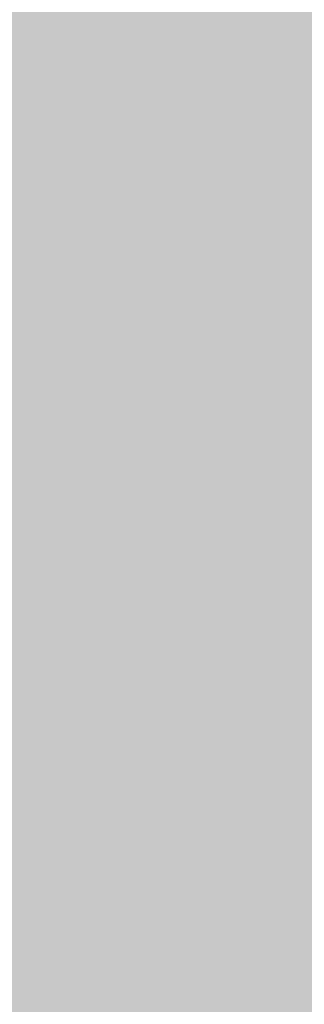
# Model space of a CAD drawing. Units: millimetres. Extents: x -22994 to 29398, y -19990 to 20176.
# Tile 81 of 135: x 225.814 to 226.355, y 85.199 to 87.071. Entities that reach past the tile are written whole.
import ezdxf
from ezdxf import colors
from ezdxf.entities.mleader import LeaderData, LeaderLine
from ezdxf.math import Vec2, Vec3

# ---------------------------------------------------------------- set-up
doc = ezdxf.new("R2010")
doc.units = ezdxf.units.MM
doc.header["$MEASUREMENT"] = 0
doc.layers.add('M-ANNO-TEXT', color=7, linetype='Continuous', lineweight=25)
doc.layers.add('M-DIMS', color=2, linetype='Continuous', lineweight=18)
doc.styles.get("Standard").update_dxf_attribs({"font": 'arial.ttf'})
doc.dimstyles.get("Standard").update_dxf_attribs({"dimtxt": 0.18, "dimasz": 10000, "dimexe": 0.18, "dimexo": 0.0625, "dimgap": 0.09, "dimtad": 0, "dimtih": 1, "dimtoh": 1, "dimdec": 0, "dimzin": 0, "dimdsep": 46, "dimtxsty": 'Standard', "dimcen": 0.09, "dimadec": 0, "dimazin": 0, "dimtfac": 1, "dimtdec": 0, "dimtofl": 0, "dimtmove": 0, "dimatfit": 3, "dimfxl": 1, "dimtolj": 1, "dimtzin": 0, "dimlwd": 30, "dimarcsym": 0})

# ---------------------------------------------------------------- blocks, each defined once
blk = doc.blocks.new('*D2')
at = {"layer": 'Defpoints', "color": 0, "transparency": 16777216}
for p in [(6.6773, 10.2713), (290.852, 10.2713), (290.852, -5.0787)]:
    blk.add_point(p, dxfattribs=at)
at = {"layer": 'M-DIMS', "color": 0, "lineweight": -2, "transparency": 16777216}
for p, q in [((6.6773, 10.2088), (6.6773, -5.2587)), ((290.852, 10.2088), (290.852, -5.2587))]:
    blk.add_line(p, q, dxfattribs=at)
at = {"layer": 'M-DIMS', "color": 0, "lineweight": 30, "transparency": 16777216}
for p, q in [((-9993.3227, -5.0787), (-19993.3227, -5.0787)), ((10290.852, -5.0787), (20290.852, -5.0787))]:
    blk.add_line(p, q, dxfattribs=at)
at = {"layer": 'M-DIMS', "color": 0, "transparency": 16777216}
for points in [[(-9993.3227, 1661.5879), (-9993.3227, -1671.7454), (6.6773, -5.0787)], [(10290.852, 1661.5879), (10290.852, -1671.7454), (290.852, -5.0787)]]:
    blk.add_solid(points, dxfattribs=at)
at = {"layer": 'M-DIMS', "color": 0, "transparency": 16777216, "insert": (148.7647, -5.0787), "char_height": 0.18, "attachment_point": 5}
blk.add_mtext('\\A1;284.2', dxfattribs=at)
blk = doc.blocks.new('*D3')
at = {"layer": 'Defpoints', "color": 0, "transparency": 16777216}
for p in [(110.2647, 204.1654), (110.2647, 176.3662), (95.8327, 127.967)]:
    blk.add_point(p, dxfattribs=at)
at = {"layer": 'M-DIMS', "color": 0, "lineweight": -2, "transparency": 16777216}
for p, q in [((95.8327, 128.0295), (95.8327, 204.3454)), ((110.2647, 176.4287), (110.2647, 204.3454))]:
    blk.add_line(p, q, dxfattribs=at)
at = {"layer": 'M-DIMS', "color": 0, "lineweight": 30, "transparency": 16777216}
for p, q in [((-9904.1673, 204.1654), (-19904.1673, 204.1654)), ((10110.2647, 204.1654), (20110.2647, 204.1654))]:
    blk.add_line(p, q, dxfattribs=at)
at = {"layer": 'M-DIMS', "color": 0, "transparency": 16777216}
for points in [[(-9904.1673, 1870.8321), (-9904.1673, -1462.5013), (95.8327, 204.1654)], [(10110.2647, 1870.8321), (10110.2647, -1462.5013), (110.2647, 204.1654)]]:
    blk.add_solid(points, dxfattribs=at)
at = {"layer": 'M-DIMS', "color": 0, "transparency": 16777216, "insert": (103.0487, 204.1654), "char_height": 0.18, "attachment_point": 5}
blk.add_mtext('\\A1;14.432', dxfattribs=at)
blk = doc.blocks.new('*D4')
at = {"layer": 'Defpoints', "color": 0, "transparency": 16777216}
for p in [(116.2647, 204.1654), (110.2647, 176.3662), (116.2647, 176.3662)]:
    blk.add_point(p, dxfattribs=at)
at = {"layer": 'M-DIMS', "color": 0, "lineweight": -2, "transparency": 16777216}
for p, q in [((110.2647, 176.4287), (110.2647, 204.3454)), ((116.2647, 176.4287), (116.2647, 204.3454))]:
    blk.add_line(p, q, dxfattribs=at)
at = {"layer": 'M-DIMS', "color": 0, "lineweight": 30, "transparency": 16777216}
for p, q in [((-9889.7353, 204.1654), (-19889.7353, 204.1654)), ((10116.2647, 204.1654), (20116.2647, 204.1654))]:
    blk.add_line(p, q, dxfattribs=at)
at = {"layer": 'M-DIMS', "color": 0, "transparency": 16777216}
for points in [[(-9889.7353, 1870.8321), (-9889.7353, -1462.5013), (110.2647, 204.1654)], [(10116.2647, 1870.8321), (10116.2647, -1462.5013), (116.2647, 204.1654)]]:
    blk.add_solid(points, dxfattribs=at)
at = {"layer": 'M-DIMS', "color": 0, "transparency": 16777216, "insert": (113.2647, 204.1654), "char_height": 0.18, "attachment_point": 5}
blk.add_mtext('\\A1;6', dxfattribs=at)
blk = doc.blocks.new('*D5')
at = {"layer": 'Defpoints', "color": 0, "transparency": 16777216}
for p in [(181.2647, 204.1654), (116.2647, 176.3662), (181.2647, 176.3662)]:
    blk.add_point(p, dxfattribs=at)
at = {"layer": 'M-DIMS', "color": 0, "lineweight": -2, "transparency": 16777216}
for p, q in [((116.2647, 176.4287), (116.2647, 204.3454)), ((181.2647, 176.4287), (181.2647, 204.3454))]:
    blk.add_line(p, q, dxfattribs=at)
at = {"layer": 'M-DIMS', "color": 0, "lineweight": 30, "transparency": 16777216}
for p, q in [((-9883.7353, 204.1654), (-19883.7353, 204.1654)), ((10181.2647, 204.1654), (20181.2647, 204.1654))]:
    blk.add_line(p, q, dxfattribs=at)
at = {"layer": 'M-DIMS', "color": 0, "transparency": 16777216}
for points in [[(-9883.7353, 1870.8321), (-9883.7353, -1462.5013), (116.2647, 204.1654)], [(10181.2647, 1870.8321), (10181.2647, -1462.5013), (181.2647, 204.1654)]]:
    blk.add_solid(points, dxfattribs=at)
at = {"layer": 'M-DIMS', "color": 0, "transparency": 16777216, "insert": (148.7647, 204.1654), "char_height": 0.18, "attachment_point": 5}
blk.add_mtext('\\A1;65', dxfattribs=at)
blk = doc.blocks.new('*D6')
at = {"layer": 'Defpoints', "color": 0, "transparency": 16777216}
for p in [(187.2647, 204.1654), (181.2647, 176.3662), (187.2647, 176.3662)]:
    blk.add_point(p, dxfattribs=at)
at = {"layer": 'M-DIMS', "color": 0, "lineweight": -2, "transparency": 16777216}
for p, q in [((181.2647, 176.4287), (181.2647, 204.3454)), ((187.2647, 176.4287), (187.2647, 204.3454))]:
    blk.add_line(p, q, dxfattribs=at)
at = {"layer": 'M-DIMS', "color": 0, "lineweight": 30, "transparency": 16777216}
for p, q in [((-9818.7353, 204.1654), (-19818.7353, 204.1654)), ((10187.2647, 204.1654), (20187.2647, 204.1654))]:
    blk.add_line(p, q, dxfattribs=at)
at = {"layer": 'M-DIMS', "color": 0, "transparency": 16777216}
for points in [[(-9818.7353, 1870.8321), (-9818.7353, -1462.5013), (181.2647, 204.1654)], [(10187.2647, 1870.8321), (10187.2647, -1462.5013), (187.2647, 204.1654)]]:
    blk.add_solid(points, dxfattribs=at)
at = {"layer": 'M-DIMS', "color": 0, "transparency": 16777216, "insert": (184.2647, 204.1654), "char_height": 0.18, "attachment_point": 5}
blk.add_mtext('\\A1;6', dxfattribs=at)
blk = doc.blocks.new('*D7')
at = {"layer": 'Defpoints', "color": 0, "transparency": 16777216}
for p in [(201.6967, 204.1654), (187.2647, 176.3662), (201.6967, 127.967)]:
    blk.add_point(p, dxfattribs=at)
at = {"layer": 'M-DIMS', "color": 0, "lineweight": -2, "transparency": 16777216}
for p, q in [((187.2647, 176.4287), (187.2647, 204.3454)), ((201.6967, 128.0295), (201.6967, 204.3454))]:
    blk.add_line(p, q, dxfattribs=at)
at = {"layer": 'M-DIMS', "color": 0, "lineweight": 30, "transparency": 16777216}
for p, q in [((-9812.7353, 204.1654), (-19812.7353, 204.1654)), ((10201.6967, 204.1654), (20201.6967, 204.1654))]:
    blk.add_line(p, q, dxfattribs=at)
at = {"layer": 'M-DIMS', "color": 0, "transparency": 16777216}
for points in [[(-9812.7353, 1870.8321), (-9812.7353, -1462.5013), (187.2647, 204.1654)], [(10201.6967, 1870.8321), (10201.6967, -1462.5013), (201.6967, 204.1654)]]:
    blk.add_solid(points, dxfattribs=at)
at = {"layer": 'M-DIMS', "color": 0, "transparency": 16777216, "insert": (194.4807, 204.1654), "char_height": 0.18, "attachment_point": 5}
blk.add_mtext('\\A1;14.432', dxfattribs=at)
blk = doc.blocks.new('*D8')
at = {"layer": 'Defpoints', "color": 0, "transparency": 16777216}
for p in [(227.6485, 204.1654), (227.6485, 146.7296), (201.6967, 127.967)]:
    blk.add_point(p, dxfattribs=at)
at = {"layer": 'M-DIMS', "color": 0, "lineweight": -2, "transparency": 16777216}
for p, q in [((201.6967, 128.0295), (201.6967, 204.3454)), ((227.6485, 146.7921), (227.6485, 204.3454))]:
    blk.add_line(p, q, dxfattribs=at)
at = {"layer": 'M-DIMS', "color": 0, "lineweight": 30, "transparency": 16777216}
for p, q in [((-9798.3033, 204.1654), (-19798.3033, 204.1654)), ((10227.6485, 204.1654), (20227.6485, 204.1654))]:
    blk.add_line(p, q, dxfattribs=at)
at = {"layer": 'M-DIMS', "color": 0, "transparency": 16777216}
for points in [[(-9798.3033, 1870.8321), (-9798.3033, -1462.5013), (201.6967, 204.1654)], [(10227.6485, 1870.8321), (10227.6485, -1462.5013), (227.6485, 204.1654)]]:
    blk.add_solid(points, dxfattribs=at)
at = {"layer": 'M-DIMS', "color": 0, "transparency": 16777216, "insert": (214.6726, 204.1654), "char_height": 0.18, "attachment_point": 5}
blk.add_mtext('\\A1;25.95', dxfattribs=at)
blk = doc.blocks.new('*D9')
at = {"layer": 'Defpoints', "color": 0, "transparency": 16777216}
for p in [(187.2647, 176.3662), (306.202, 176.3662), (290.852, 10.2713)]:
    blk.add_point(p, dxfattribs=at)
at = {"layer": 'M-DIMS', "color": 0, "lineweight": 30, "transparency": 16777216}
for p, q in [((306.202, 10176.3662), (306.202, 20176.3662)), ((306.202, -9989.7287), (306.202, -19989.7287))]:
    blk.add_line(p, q, dxfattribs=at)
at = {"layer": 'M-DIMS', "color": 0, "lineweight": -2, "transparency": 16777216}
for p, q in [((187.3272, 176.3662), (306.382, 176.3662)), ((290.9145, 10.2713), (306.382, 10.2713))]:
    blk.add_line(p, q, dxfattribs=at)
at = {"layer": 'M-DIMS', "color": 0, "transparency": 16777216}
for points in [[(-1360.4646, 10176.3662), (1972.8687, 10176.3662), (306.202, 176.3662)], [(-1360.4646, -9989.7287), (1972.8687, -9989.7287), (306.202, 10.2713)]]:
    blk.add_solid(points, dxfattribs=at)
at = {"layer": 'M-DIMS', "color": 0, "transparency": 16777216, "insert": (306.202, 93.3187), "char_height": 0.18, "attachment_point": 5}
blk.add_mtext('\\A1;166.1', dxfattribs=at)
blk = doc.blocks.new('*D10')
at = {"layer": 'Defpoints', "color": 0, "transparency": 16777216}
for p in [(125.6498, 136.0713), (133.3459, 136.0713), (133.3459, -5.0787)]:
    blk.add_point(p, dxfattribs=at)
at = {"layer": 'M-DIMS', "color": 0, "lineweight": -2, "transparency": 16777216}
for p, q in [((125.6498, 136.0088), (125.6498, -5.2587)), ((133.3459, 136.0088), (133.3459, -5.2587))]:
    blk.add_line(p, q, dxfattribs=at)
at = {"layer": 'M-DIMS', "color": 0, "lineweight": 30, "transparency": 16777216}
for p, q in [((-9874.3502, -5.0787), (-19874.3502, -5.0787)), ((10133.3459, -5.0787), (20133.3459, -5.0787))]:
    blk.add_line(p, q, dxfattribs=at)
at = {"layer": 'M-DIMS', "color": 0, "transparency": 16777216}
for points in [[(-9874.3502, 1661.5879), (-9874.3502, -1671.7454), (125.6498, -5.0787)], [(10133.3459, 1661.5879), (10133.3459, -1671.7454), (133.3459, -5.0787)]]:
    blk.add_solid(points, dxfattribs=at)
at = {"layer": 'M-DIMS', "color": 0, "transparency": 16777216, "insert": (129.4978, -5.0787), "char_height": 0.18, "attachment_point": 5}
blk.add_mtext('\\A1;7.696', dxfattribs=at)
blk = doc.blocks.new('*D11')
at = {"layer": 'Defpoints', "color": 0, "transparency": 16777216}
for p in [(133.3459, 136.0713), (135.6498, 136.0713), (135.6498, -5.0787)]:
    blk.add_point(p, dxfattribs=at)
at = {"layer": 'M-DIMS', "color": 0, "lineweight": -2, "transparency": 16777216}
for p, q in [((133.3459, 136.0088), (133.3459, -5.2587)), ((135.6498, 136.0088), (135.6498, -5.2587))]:
    blk.add_line(p, q, dxfattribs=at)
at = {"layer": 'M-DIMS', "color": 0, "lineweight": 30, "transparency": 16777216}
for p, q in [((-9866.6541, -5.0787), (-19866.6541, -5.0787)), ((10135.6498, -5.0787), (20135.6498, -5.0787))]:
    blk.add_line(p, q, dxfattribs=at)
at = {"layer": 'M-DIMS', "color": 0, "transparency": 16777216}
for points in [[(-9866.6541, 1661.5879), (-9866.6541, -1671.7454), (133.3459, -5.0787)], [(10135.6498, 1661.5879), (10135.6498, -1671.7454), (135.6498, -5.0787)]]:
    blk.add_solid(points, dxfattribs=at)
at = {"layer": 'M-DIMS', "color": 0, "transparency": 16777216, "insert": (134.4978, -5.0787), "char_height": 0.18, "attachment_point": 5}
blk.add_mtext('\\A1;2.304', dxfattribs=at)
blk = doc.blocks.new('*D12')
at = {"layer": 'Defpoints', "color": 0, "transparency": 16777216}
for p in [(135.6498, 136.0713), (145.6498, 136.0713), (145.6498, -5.0787)]:
    blk.add_point(p, dxfattribs=at)
at = {"layer": 'M-DIMS', "color": 0, "lineweight": -2, "transparency": 16777216}
for p, q in [((135.6498, 136.0088), (135.6498, -5.2587)), ((145.6498, 136.0088), (145.6498, -5.2587))]:
    blk.add_line(p, q, dxfattribs=at)
at = {"layer": 'M-DIMS', "color": 0, "lineweight": 30, "transparency": 16777216}
for p, q in [((-9864.3502, -5.0787), (-19864.3502, -5.0787)), ((10145.6498, -5.0787), (20145.6498, -5.0787))]:
    blk.add_line(p, q, dxfattribs=at)
at = {"layer": 'M-DIMS', "color": 0, "transparency": 16777216}
for points in [[(-9864.3502, 1661.5879), (-9864.3502, -1671.7454), (135.6498, -5.0787)], [(10145.6498, 1661.5879), (10145.6498, -1671.7454), (145.6498, -5.0787)]]:
    blk.add_solid(points, dxfattribs=at)
at = {"layer": 'M-DIMS', "color": 0, "transparency": 16777216, "insert": (140.6498, -5.0787), "char_height": 0.18, "attachment_point": 5}
blk.add_mtext('\\A1;10', dxfattribs=at)
blk = doc.blocks.new('*D13')
at = {"layer": 'Defpoints', "color": 0, "transparency": 16777216}
for p in [(145.6498, 136.0713), (155.6498, 136.0713), (155.6498, -5.0787)]:
    blk.add_point(p, dxfattribs=at)
at = {"layer": 'M-DIMS', "color": 0, "lineweight": -2, "transparency": 16777216}
for p, q in [((145.6498, 136.0088), (145.6498, -5.2587)), ((155.6498, 136.0088), (155.6498, -5.2587))]:
    blk.add_line(p, q, dxfattribs=at)
at = {"layer": 'M-DIMS', "color": 0, "lineweight": 30, "transparency": 16777216}
for p, q in [((-9854.3502, -5.0787), (-19854.3502, -5.0787)), ((10155.6498, -5.0787), (20155.6498, -5.0787))]:
    blk.add_line(p, q, dxfattribs=at)
at = {"layer": 'M-DIMS', "color": 0, "transparency": 16777216}
for points in [[(-9854.3502, 1661.5879), (-9854.3502, -1671.7454), (145.6498, -5.0787)], [(10155.6498, 1661.5879), (10155.6498, -1671.7454), (155.6498, -5.0787)]]:
    blk.add_solid(points, dxfattribs=at)
at = {"layer": 'M-DIMS', "color": 0, "transparency": 16777216, "insert": (150.6498, -5.0787), "char_height": 0.18, "attachment_point": 5}
blk.add_mtext('\\A1;10', dxfattribs=at)
blk = doc.blocks.new('*D14')
at = {"layer": 'Defpoints', "color": 0, "transparency": 16777216}
for p in [(155.6498, 136.0713), (165.6498, 136.0713), (165.6498, -5.0787)]:
    blk.add_point(p, dxfattribs=at)
at = {"layer": 'M-DIMS', "color": 0, "lineweight": -2, "transparency": 16777216}
for p, q in [((155.6498, 136.0088), (155.6498, -5.2587)), ((165.6498, 136.0088), (165.6498, -5.2587))]:
    blk.add_line(p, q, dxfattribs=at)
at = {"layer": 'M-DIMS', "color": 0, "lineweight": 30, "transparency": 16777216}
for p, q in [((-9844.3502, -5.0787), (-19844.3502, -5.0787)), ((10165.6498, -5.0787), (20165.6498, -5.0787))]:
    blk.add_line(p, q, dxfattribs=at)
at = {"layer": 'M-DIMS', "color": 0, "transparency": 16777216}
for points in [[(-9844.3502, 1661.5879), (-9844.3502, -1671.7454), (155.6498, -5.0787)], [(10165.6498, 1661.5879), (10165.6498, -1671.7454), (165.6498, -5.0787)]]:
    blk.add_solid(points, dxfattribs=at)
at = {"layer": 'M-DIMS', "color": 0, "transparency": 16777216, "insert": (160.6498, -5.0787), "char_height": 0.18, "attachment_point": 5}
blk.add_mtext('\\A1;10', dxfattribs=at)
blk = doc.blocks.new('*D15')
at = {"layer": 'Defpoints', "color": 0, "transparency": 16777216}
for p in [(173.3459, 154.788), (173.3459, 136.0713), (306.202, 136.0713)]:
    blk.add_point(p, dxfattribs=at)
at = {"layer": 'M-DIMS', "color": 0, "lineweight": 30, "transparency": 16777216}
for p, q in [((306.202, 10154.788), (306.202, 20154.788)), ((306.202, -9863.9287), (306.202, -19863.9287))]:
    blk.add_line(p, q, dxfattribs=at)
at = {"layer": 'M-DIMS', "color": 0, "lineweight": -2, "transparency": 16777216}
for p, q in [((173.4084, 154.788), (306.382, 154.788)), ((173.4084, 136.0713), (306.382, 136.0713))]:
    blk.add_line(p, q, dxfattribs=at)
at = {"layer": 'M-DIMS', "color": 0, "transparency": 16777216}
for points in [[(-1360.4646, 10154.788), (1972.8687, 10154.788), (306.202, 154.788)], [(-1360.4646, -9863.9287), (1972.8687, -9863.9287), (306.202, 136.0713)]]:
    blk.add_solid(points, dxfattribs=at)
at = {"layer": 'M-DIMS', "color": 0, "transparency": 16777216, "insert": (306.202, 145.4297), "char_height": 0.18, "attachment_point": 5}
blk.add_mtext('\\A1;18.717', dxfattribs=at)
blk = doc.blocks.new('*D16')
at = {"layer": 'Defpoints', "color": 0, "transparency": 16777216}
for p in [(120.1702, 204.1654), (110.4658, 48.0349), (120.1702, 48.0349)]:
    blk.add_point(p, dxfattribs=at)
at = {"layer": 'M-DIMS', "color": 0, "lineweight": -2, "transparency": 16777216}
for p, q in [((110.4658, 48.0974), (110.4658, 204.3454)), ((120.1702, 48.0974), (120.1702, 204.3454))]:
    blk.add_line(p, q, dxfattribs=at)
at = {"layer": 'M-DIMS', "color": 0, "lineweight": 30, "transparency": 16777216}
for p, q in [((-9889.5342, 204.1654), (-19889.5342, 204.1654)), ((10120.1702, 204.1654), (20120.1702, 204.1654))]:
    blk.add_line(p, q, dxfattribs=at)
at = {"layer": 'M-DIMS', "color": 0, "transparency": 16777216}
for points in [[(-9889.5342, 1870.8321), (-9889.5342, -1462.5013), (110.4658, 204.1654)], [(10120.1702, 1870.8321), (10120.1702, -1462.5013), (120.1702, 204.1654)]]:
    blk.add_solid(points, dxfattribs=at)
at = {"layer": 'M-DIMS', "color": 0, "transparency": 16777216, "insert": (115.318, 204.1654), "char_height": 0.18, "attachment_point": 5}
blk.add_mtext('\\A1;9.704', dxfattribs=at)
blk = doc.blocks.new('*D17')
at = {"layer": 'Defpoints', "color": 0, "transparency": 16777216}
for p in [(126.1702, 204.1654), (120.1702, 48.0349), (126.1702, 48.0349)]:
    blk.add_point(p, dxfattribs=at)
at = {"layer": 'M-DIMS', "color": 0, "lineweight": -2, "transparency": 16777216}
for p, q in [((120.1702, 48.0974), (120.1702, 204.3454)), ((126.1702, 48.0974), (126.1702, 204.3454))]:
    blk.add_line(p, q, dxfattribs=at)
at = {"layer": 'M-DIMS', "color": 0, "lineweight": 30, "transparency": 16777216}
for p, q in [((-9879.8298, 204.1654), (-19879.8298, 204.1654)), ((10126.1702, 204.1654), (20126.1702, 204.1654))]:
    blk.add_line(p, q, dxfattribs=at)
at = {"layer": 'M-DIMS', "color": 0, "transparency": 16777216}
for points in [[(-9879.8298, 1870.8321), (-9879.8298, -1462.5013), (120.1702, 204.1654)], [(10126.1702, 1870.8321), (10126.1702, -1462.5013), (126.1702, 204.1654)]]:
    blk.add_solid(points, dxfattribs=at)
at = {"layer": 'M-DIMS', "color": 0, "transparency": 16777216, "insert": (123.1702, 204.1654), "char_height": 0.18, "attachment_point": 5}
blk.add_mtext('\\A1;6', dxfattribs=at)
blk = doc.blocks.new('*D18')
at = {"layer": 'Defpoints', "color": 0, "transparency": 16777216}
for p in [(132.1702, 204.1654), (126.1702, 48.0349), (132.1702, 48.0349)]:
    blk.add_point(p, dxfattribs=at)
at = {"layer": 'M-DIMS', "color": 0, "lineweight": -2, "transparency": 16777216}
for p, q in [((126.1702, 48.0974), (126.1702, 204.3454)), ((132.1702, 48.0974), (132.1702, 204.3454))]:
    blk.add_line(p, q, dxfattribs=at)
at = {"layer": 'M-DIMS', "color": 0, "lineweight": 30, "transparency": 16777216}
for p, q in [((-9873.8298, 204.1654), (-19873.8298, 204.1654)), ((10132.1702, 204.1654), (20132.1702, 204.1654))]:
    blk.add_line(p, q, dxfattribs=at)
at = {"layer": 'M-DIMS', "color": 0, "transparency": 16777216}
for points in [[(-9873.8298, 1870.8321), (-9873.8298, -1462.5013), (126.1702, 204.1654)], [(10132.1702, 1870.8321), (10132.1702, -1462.5013), (132.1702, 204.1654)]]:
    blk.add_solid(points, dxfattribs=at)
at = {"layer": 'M-DIMS', "color": 0, "transparency": 16777216, "insert": (129.1702, 204.1654), "char_height": 0.18, "attachment_point": 5}
blk.add_mtext('\\A1;6', dxfattribs=at)
blk = doc.blocks.new('*D19')
at = {"layer": 'Defpoints', "color": 0, "transparency": 16777216}
for p in [(138.1702, 204.1654), (132.1702, 48.0349), (138.1702, 48.0349)]:
    blk.add_point(p, dxfattribs=at)
at = {"layer": 'M-DIMS', "color": 0, "lineweight": -2, "transparency": 16777216}
for p, q in [((132.1702, 48.0974), (132.1702, 204.3454)), ((138.1702, 48.0974), (138.1702, 204.3454))]:
    blk.add_line(p, q, dxfattribs=at)
at = {"layer": 'M-DIMS', "color": 0, "lineweight": 30, "transparency": 16777216}
for p, q in [((-9867.8298, 204.1654), (-19867.8298, 204.1654)), ((10138.1702, 204.1654), (20138.1702, 204.1654))]:
    blk.add_line(p, q, dxfattribs=at)
at = {"layer": 'M-DIMS', "color": 0, "transparency": 16777216}
for points in [[(-9867.8298, 1870.8321), (-9867.8298, -1462.5013), (132.1702, 204.1654)], [(10138.1702, 1870.8321), (10138.1702, -1462.5013), (138.1702, 204.1654)]]:
    blk.add_solid(points, dxfattribs=at)
at = {"layer": 'M-DIMS', "color": 0, "transparency": 16777216, "insert": (135.1702, 204.1654), "char_height": 0.18, "attachment_point": 5}
blk.add_mtext('\\A1;6', dxfattribs=at)
blk = doc.blocks.new('*D20')
at = {"layer": 'Defpoints', "color": 0, "transparency": 16777216}
for p in [(144.1702, 204.1654), (138.1702, 48.0349), (144.1702, 48.0349)]:
    blk.add_point(p, dxfattribs=at)
at = {"layer": 'M-DIMS', "color": 0, "lineweight": -2, "transparency": 16777216}
for p, q in [((138.1702, 48.0974), (138.1702, 204.3454)), ((144.1702, 48.0974), (144.1702, 204.3454))]:
    blk.add_line(p, q, dxfattribs=at)
at = {"layer": 'M-DIMS', "color": 0, "lineweight": 30, "transparency": 16777216}
for p, q in [((-9861.8298, 204.1654), (-19861.8298, 204.1654)), ((10144.1702, 204.1654), (20144.1702, 204.1654))]:
    blk.add_line(p, q, dxfattribs=at)
at = {"layer": 'M-DIMS', "color": 0, "transparency": 16777216}
for points in [[(-9861.8298, 1870.8321), (-9861.8298, -1462.5013), (138.1702, 204.1654)], [(10144.1702, 1870.8321), (10144.1702, -1462.5013), (144.1702, 204.1654)]]:
    blk.add_solid(points, dxfattribs=at)
at = {"layer": 'M-DIMS', "color": 0, "transparency": 16777216, "insert": (141.1702, 204.1654), "char_height": 0.18, "attachment_point": 5}
blk.add_mtext('\\A1;6', dxfattribs=at)
blk = doc.blocks.new('*D21')
at = {"layer": 'Defpoints', "color": 0, "transparency": 16777216}
for p in [(149.1157, 204.1654), (144.1702, 48.0349), (149.1157, 48.0349)]:
    blk.add_point(p, dxfattribs=at)
at = {"layer": 'M-DIMS', "color": 0, "lineweight": -2, "transparency": 16777216}
for p, q in [((144.1702, 48.0974), (144.1702, 204.3454)), ((149.1157, 48.0974), (149.1157, 204.3454))]:
    blk.add_line(p, q, dxfattribs=at)
at = {"layer": 'M-DIMS', "color": 0, "lineweight": 30, "transparency": 16777216}
for p, q in [((-9855.8298, 204.1654), (-19855.8298, 204.1654)), ((10149.1157, 204.1654), (20149.1157, 204.1654))]:
    blk.add_line(p, q, dxfattribs=at)
at = {"layer": 'M-DIMS', "color": 0, "transparency": 16777216}
for points in [[(-9855.8298, 1870.8321), (-9855.8298, -1462.5013), (144.1702, 204.1654)], [(10149.1157, 1870.8321), (10149.1157, -1462.5013), (149.1157, 204.1654)]]:
    blk.add_solid(points, dxfattribs=at)
at = {"layer": 'M-DIMS', "color": 0, "transparency": 16777216, "insert": (146.6429, 204.1654), "char_height": 0.18, "attachment_point": 5}
blk.add_mtext('\\A1;4.945', dxfattribs=at)
blk = doc.blocks.new('*D22')
at = {"layer": 'Defpoints', "color": 0, "transparency": 16777216}
for p in [(149.1157, 30.9895), (155.1157, 30.9895), (155.1157, -5.0787)]:
    blk.add_point(p, dxfattribs=at)
at = {"layer": 'M-DIMS', "color": 0, "lineweight": -2, "transparency": 16777216}
for p, q in [((149.1157, 30.927), (149.1157, -5.2587)), ((155.1157, 30.927), (155.1157, -5.2587))]:
    blk.add_line(p, q, dxfattribs=at)
at = {"layer": 'M-DIMS', "color": 0, "lineweight": 30, "transparency": 16777216}
for p, q in [((-9850.8843, -5.0787), (-19850.8843, -5.0787)), ((10155.1157, -5.0787), (20155.1157, -5.0787))]:
    blk.add_line(p, q, dxfattribs=at)
at = {"layer": 'M-DIMS', "color": 0, "transparency": 16777216}
for points in [[(-9850.8843, 1661.5879), (-9850.8843, -1671.7454), (149.1157, -5.0787)], [(10155.1157, 1661.5879), (10155.1157, -1671.7454), (155.1157, -5.0787)]]:
    blk.add_solid(points, dxfattribs=at)
at = {"layer": 'M-DIMS', "color": 0, "transparency": 16777216, "insert": (152.1157, -5.0787), "char_height": 0.18, "attachment_point": 5}
blk.add_mtext('\\A1;6', dxfattribs=at)
blk = doc.blocks.new('*D23')
at = {"layer": 'Defpoints', "color": 0, "transparency": 16777216}
for p in [(155.1157, 30.9895), (161.1157, 30.9895), (161.1157, -5.0787)]:
    blk.add_point(p, dxfattribs=at)
at = {"layer": 'M-DIMS', "color": 0, "lineweight": -2, "transparency": 16777216}
for p, q in [((155.1157, 30.927), (155.1157, -5.2587)), ((161.1157, 30.927), (161.1157, -5.2587))]:
    blk.add_line(p, q, dxfattribs=at)
at = {"layer": 'M-DIMS', "color": 0, "lineweight": 30, "transparency": 16777216}
for p, q in [((-9844.8843, -5.0787), (-19844.8843, -5.0787)), ((10161.1157, -5.0787), (20161.1157, -5.0787))]:
    blk.add_line(p, q, dxfattribs=at)
at = {"layer": 'M-DIMS', "color": 0, "transparency": 16777216}
for points in [[(-9844.8843, 1661.5879), (-9844.8843, -1671.7454), (155.1157, -5.0787)], [(10161.1157, 1661.5879), (10161.1157, -1671.7454), (161.1157, -5.0787)]]:
    blk.add_solid(points, dxfattribs=at)
at = {"layer": 'M-DIMS', "color": 0, "transparency": 16777216, "insert": (158.1157, -5.0787), "char_height": 0.18, "attachment_point": 5}
blk.add_mtext('\\A1;6', dxfattribs=at)
blk = doc.blocks.new('*D24')
at = {"layer": 'Defpoints', "color": 0, "transparency": 16777216}
for p in [(161.1157, 30.9895), (166.4387, 30.9895), (166.4387, -5.0787)]:
    blk.add_point(p, dxfattribs=at)
at = {"layer": 'M-DIMS', "color": 0, "lineweight": -2, "transparency": 16777216}
for p, q in [((161.1157, 30.927), (161.1157, -5.2587)), ((166.4387, 30.927), (166.4387, -5.2587))]:
    blk.add_line(p, q, dxfattribs=at)
at = {"layer": 'M-DIMS', "color": 0, "lineweight": 30, "transparency": 16777216}
for p, q in [((-9838.8843, -5.0787), (-19838.8843, -5.0787)), ((10166.4387, -5.0787), (20166.4387, -5.0787))]:
    blk.add_line(p, q, dxfattribs=at)
at = {"layer": 'M-DIMS', "color": 0, "transparency": 16777216}
for points in [[(-9838.8843, 1661.5879), (-9838.8843, -1671.7454), (161.1157, -5.0787)], [(10166.4387, 1661.5879), (10166.4387, -1671.7454), (166.4387, -5.0787)]]:
    blk.add_solid(points, dxfattribs=at)
at = {"layer": 'M-DIMS', "color": 0, "transparency": 16777216, "insert": (163.7772, -5.0787), "char_height": 0.18, "attachment_point": 5}
blk.add_mtext('\\A1;5.323', dxfattribs=at)
blk = doc.blocks.new('*D25')
at = {"layer": 'Defpoints', "color": 0, "transparency": 16777216}
for p in [(166.4387, 30.9895), (172.4387, 30.9895), (172.4387, -5.0787)]:
    blk.add_point(p, dxfattribs=at)
at = {"layer": 'M-DIMS', "color": 0, "lineweight": -2, "transparency": 16777216}
for p, q in [((166.4387, 30.927), (166.4387, -5.2587)), ((172.4387, 30.927), (172.4387, -5.2587))]:
    blk.add_line(p, q, dxfattribs=at)
at = {"layer": 'M-DIMS', "color": 0, "lineweight": 30, "transparency": 16777216}
for p, q in [((-9833.5613, -5.0787), (-19833.5613, -5.0787)), ((10172.4387, -5.0787), (20172.4387, -5.0787))]:
    blk.add_line(p, q, dxfattribs=at)
at = {"layer": 'M-DIMS', "color": 0, "transparency": 16777216}
for points in [[(-9833.5613, 1661.5879), (-9833.5613, -1671.7454), (166.4387, -5.0787)], [(10172.4387, 1661.5879), (10172.4387, -1671.7454), (172.4387, -5.0787)]]:
    blk.add_solid(points, dxfattribs=at)
at = {"layer": 'M-DIMS', "color": 0, "transparency": 16777216, "insert": (169.4387, -5.0787), "char_height": 0.18, "attachment_point": 5}
blk.add_mtext('\\A1;6', dxfattribs=at)
blk = doc.blocks.new('*D26')
at = {"layer": 'Defpoints', "color": 0, "transparency": 16777216}
for p in [(172.4387, 30.9895), (178.4387, 30.9895), (178.4387, -5.0787)]:
    blk.add_point(p, dxfattribs=at)
at = {"layer": 'M-DIMS', "color": 0, "lineweight": -2, "transparency": 16777216}
for p, q in [((172.4387, 30.927), (172.4387, -5.2587)), ((178.4387, 30.927), (178.4387, -5.2587))]:
    blk.add_line(p, q, dxfattribs=at)
at = {"layer": 'M-DIMS', "color": 0, "lineweight": 30, "transparency": 16777216}
for p, q in [((-9827.5613, -5.0787), (-19827.5613, -5.0787)), ((10178.4387, -5.0787), (20178.4387, -5.0787))]:
    blk.add_line(p, q, dxfattribs=at)
at = {"layer": 'M-DIMS', "color": 0, "transparency": 16777216}
for points in [[(-9827.5613, 1661.5879), (-9827.5613, -1671.7454), (172.4387, -5.0787)], [(10178.4387, 1661.5879), (10178.4387, -1671.7454), (178.4387, -5.0787)]]:
    blk.add_solid(points, dxfattribs=at)
at = {"layer": 'M-DIMS', "color": 0, "transparency": 16777216, "insert": (175.4387, -5.0787), "char_height": 0.18, "attachment_point": 5}
blk.add_mtext('\\A1;6', dxfattribs=at)
blk = doc.blocks.new('*D27')
at = {"layer": 'Defpoints', "color": 0, "transparency": 16777216}
for p in [(178.4387, 30.9895), (188.1175, 30.9895), (188.1175, -5.0787)]:
    blk.add_point(p, dxfattribs=at)
at = {"layer": 'M-DIMS', "color": 0, "lineweight": -2, "transparency": 16777216}
for p, q in [((178.4387, 30.927), (178.4387, -5.2587)), ((188.1175, 30.927), (188.1175, -5.2587))]:
    blk.add_line(p, q, dxfattribs=at)
at = {"layer": 'M-DIMS', "color": 0, "lineweight": 30, "transparency": 16777216}
for p, q in [((-9821.5613, -5.0787), (-19821.5613, -5.0787)), ((10188.1175, -5.0787), (20188.1175, -5.0787))]:
    blk.add_line(p, q, dxfattribs=at)
at = {"layer": 'M-DIMS', "color": 0, "transparency": 16777216}
for points in [[(-9821.5613, 1661.5879), (-9821.5613, -1671.7454), (178.4387, -5.0787)], [(10188.1175, 1661.5879), (10188.1175, -1671.7454), (188.1175, -5.0787)]]:
    blk.add_solid(points, dxfattribs=at)
at = {"layer": 'M-DIMS', "color": 0, "transparency": 16777216, "insert": (183.2781, -5.0787), "char_height": 0.18, "attachment_point": 5}
blk.add_mtext('\\A1;9.679', dxfattribs=at)
blk = doc.blocks.new('*D28')
at = {"layer": 'Defpoints', "color": 0, "transparency": 16777216}
for p in [(188.1175, 48.0349), (306.202, 48.0349), (188.1175, 30.9895)]:
    blk.add_point(p, dxfattribs=at)
at = {"layer": 'M-DIMS', "color": 0, "lineweight": 30, "transparency": 16777216}
for p, q in [((306.202, 10048.0349), (306.202, 20048.0349)), ((306.202, -9969.0105), (306.202, -19969.0105))]:
    blk.add_line(p, q, dxfattribs=at)
at = {"layer": 'M-DIMS', "color": 0, "lineweight": -2, "transparency": 16777216}
for p, q in [((188.18, 48.0349), (306.382, 48.0349)), ((188.18, 30.9895), (306.382, 30.9895))]:
    blk.add_line(p, q, dxfattribs=at)
at = {"layer": 'M-DIMS', "color": 0, "transparency": 16777216}
for points in [[(-1360.4646, 10048.0349), (1972.8687, 10048.0349), (306.202, 48.0349)], [(-1360.4646, -9969.0105), (1972.8687, -9969.0105), (306.202, 30.9895)]]:
    blk.add_solid(points, dxfattribs=at)
at = {"layer": 'M-DIMS', "color": 0, "transparency": 16777216, "insert": (306.202, 39.5122), "char_height": 0.18, "attachment_point": 5}
blk.add_mtext('\\A1;17.045', dxfattribs=at)
blk = doc.blocks.new('*D29')
at = {"layer": 'Defpoints', "color": 0, "transparency": 16777216}
for p in [(36.8006, 80.045), (64.0296, 80.045)]:
    blk.add_point(p, dxfattribs=at)
at = {"layer": 'M-DIMS', "color": 0, "lineweight": -2, "transparency": 16777216}
for p, q in [((50.4151, 79.955), (50.4151, 80.135)), ((50.3251, 80.045), (50.5051, 80.045))]:
    blk.add_line(p, q, dxfattribs=at)
at = {"layer": 'M-DIMS', "color": 0, "lineweight": 30, "transparency": 16777216}
blk.add_line((20064.0296, 80.0303), (10064.0296, 80.0377), dxfattribs=at)
at = {"layer": 'M-DIMS', "color": 0, "transparency": 16777216}
blk.add_solid([(10064.0309, 1746.7043), (10064.0284, -1586.629), (64.0296, 80.045)], dxfattribs=at)
at = {"layer": 'M-DIMS', "color": 0, "transparency": 16777216, "insert": (20064.5213, 80.0303), "char_height": 0.18, "attachment_point": 5}
blk.add_mtext('\\A1;∅27.23', dxfattribs=at)
blk = doc.blocks.new('*D30')
at = {"layer": 'Defpoints', "color": 0, "transparency": 16777216}
for p in [(216.3148, 146.7291), (238.9821, 146.73)]:
    blk.add_point(p, dxfattribs=at)
at = {"layer": 'M-DIMS', "color": 0, "lineweight": 30, "transparency": 16777216}
blk.add_line((20238.9821, 147.4959), (10238.9821, 147.1129), dxfattribs=at)
at = {"layer": 'M-DIMS', "color": 0, "lineweight": -2, "transparency": 16777216}
for p, q in [((227.6485, 146.6396), (227.6485, 146.8196)), ((227.5585, 146.7296), (227.7385, 146.7296))]:
    blk.add_line(p, q, dxfattribs=at)
at = {"layer": 'M-DIMS', "color": 0, "transparency": 16777216}
blk.add_solid([(10238.9183, 1813.7796), (10239.0459, -1519.5537), (238.9821, 146.73)], dxfattribs=at)
at = {"layer": 'M-DIMS', "color": 0, "transparency": 16777216, "insert": (20239.5436, 147.4959), "char_height": 0.18, "attachment_point": 5}
blk.add_mtext('\\A1;∅22.667', dxfattribs=at)
blk = doc.blocks.new('*D31')
at = {"layer": 'Defpoints', "color": 0, "transparency": 16777216}
for p in [(223.1641, 146.7291), (232.1328, 146.73)]:
    blk.add_point(p, dxfattribs=at)
at = {"layer": 'M-DIMS', "color": 0, "lineweight": 30, "transparency": 16777216}
blk.add_line((20232.1327, 148.6656), (10232.1328, 147.6978), dxfattribs=at)
at = {"layer": 'M-DIMS', "color": 0, "lineweight": -2, "transparency": 16777216}
for p, q in [((227.6485, 146.6396), (227.6485, 146.8196)), ((227.5585, 146.7296), (227.7385, 146.7296))]:
    blk.add_line(p, q, dxfattribs=at)
at = {"layer": 'M-DIMS', "color": 0, "transparency": 16777216}
blk.add_solid([(10231.9715, 1814.3645), (10232.2941, -1518.9688), (232.1328, 146.73)], dxfattribs=at)
at = {"layer": 'M-DIMS', "color": 0, "transparency": 16777216, "insert": (20232.6245, 148.6656), "char_height": 0.18, "attachment_point": 5}
blk.add_mtext('\\A1;∅8.969', dxfattribs=at)
blk = doc.blocks.new('*D36')
at = {"layer": 'Defpoints', "color": 0, "transparency": 16777216}
for p in [(46.39, 31.3035), (46.3875, 26.5934)]:
    blk.add_point(p, dxfattribs=at)
at = {"layer": 'M-DIMS', "color": 0, "lineweight": 30, "transparency": 16777216}
for p, q in [((57.1499, 20031.3006), (51.77, 10031.302)), ((10057.1499, 20031.3006), (57.1499, 20031.3006))]:
    blk.add_line(p, q, dxfattribs=at)
at = {"layer": 'M-DIMS', "color": 0, "lineweight": -2, "transparency": 16777216}
for p, q in [((46.3887, 28.8585), (46.3887, 29.0385)), ((46.2987, 28.9485), (46.4787, 28.9485))]:
    blk.add_line(p, q, dxfattribs=at)
at = {"layer": 'M-DIMS', "color": 0, "transparency": 16777216}
blk.add_solid([(-1614.8965, 10032.1987), (1718.4364, 10030.4054), (46.39, 31.3035)], dxfattribs=at)
at = {"layer": 'M-DIMS', "color": 0, "transparency": 16777216, "insert": (10057.5542, 20031.3006), "char_height": 0.18, "attachment_point": 5}
blk.add_mtext('\\A1;∅4.71', dxfattribs=at)
blk = doc.blocks.new('*D37')
at = {"layer": 'Defpoints', "color": 0, "transparency": 16777216}
for p in [(54.8343, 118.6145), (59.4936, 118.614)]:
    blk.add_point(p, dxfattribs=at)
at = {"layer": 'M-DIMS', "color": 0, "lineweight": -2, "transparency": 16777216}
for p, q in [((57.1639, 118.5243), (57.1639, 118.7043)), ((57.0739, 118.6143), (57.2539, 118.6143))]:
    blk.add_line(p, q, dxfattribs=at)
at = {"layer": 'M-DIMS', "color": 0, "lineweight": 30, "transparency": 16777216}
blk.add_line((20059.4934, 116.2531), (10059.4935, 117.4336), dxfattribs=at)
at = {"layer": 'M-DIMS', "color": 0, "transparency": 16777216}
blk.add_solid([(10059.6902, 1784.1002), (10059.2968, -1549.2331), (59.4936, 118.614)], dxfattribs=at)
at = {"layer": 'M-DIMS', "color": 0, "transparency": 16777216, "insert": (20059.9852, 116.2531), "char_height": 0.18, "attachment_point": 5}
blk.add_mtext('\\A1;∅4.659', dxfattribs=at)

msp = doc.modelspace()

# ---------------------------------------------------------------- dimensions: what is measured, and where the dimension line sits
at = {"layer": 'M-DIMS'}
for base, p1, p2, override, picture, middle in [((306.202, 176.3662), (290.852, 10.2713), (187.2647, 176.3662), {"dimdec": 1, "dimlfac": 1, "dimrnd": 0, "dimzin": 0, "dimdsep": 46, "dimlunit": 2}, '*D9', (306.202, 93.3187)), ((306.202, 136.0713), (173.3459, 154.788), (173.3459, 136.0713), {"dimdec": 3, "dimlfac": 1, "dimrnd": 0, "dimzin": 0, "dimdsep": 46, "dimlunit": 2}, '*D15', (306.202, 145.4297)), ((306.202, 48.0349), (188.1175, 30.9895), (188.1175, 48.0349), {"dimdec": 3, "dimlfac": 1, "dimrnd": 0, "dimzin": 0, "dimdsep": 46, "dimlunit": 2}, '*D28', (306.202, 39.5122))]:
    dim = msp.add_linear_dim(base=base, p1=p1, p2=p2, angle=90, dimstyle='Standard', override=override, dxfattribs=at)
    dim.commit()
    dim.dimension.update_dxf_attribs({"geometry": picture, "text_midpoint": middle})
for p1, p2, override, picture, middle in [((46.3875, 26.5934), (46.39, 31.3035), {"dimdec": 2, "dimlfac": 1, "dimrnd": 0, "dimzin": 0, "dimdsep": 46, "dimlunit": 2}, '*D36', (10057.5542, 20031.3006)), ((223.1641, 146.7291), (232.1328, 146.73), {"dimdec": 3, "dimlfac": 1, "dimrnd": 0, "dimzin": 0, "dimdsep": 46, "dimlunit": 2}, '*D31', (20232.1327, 148.6656)), ((216.3148, 146.7291), (238.9821, 146.73), {"dimdec": 3, "dimlfac": 1, "dimrnd": 0, "dimzin": 0, "dimdsep": 46, "dimlunit": 2}, '*D30', (20238.9821, 147.4959))]:
    dim = msp.add_diameter_dim_2p(p1=p1, p2=p2, dimstyle='Standard', override=override, dxfattribs=at)
    dim.commit()
    dim.dimension.update_dxf_attribs({"geometry": picture, "text_midpoint": middle, "dimtype": 163})
for base, p1, p2, override, picture, middle in [((110.2647, 204.1654), (95.8327, 127.967), (110.2647, 176.3662), {"dimdec": 3, "dimlfac": 1, "dimrnd": 0, "dimzin": 0, "dimdsep": 46, "dimlunit": 2}, '*D3', (103.0487, 204.1654)), ((116.2647, 204.1654), (110.2647, 176.3662), (116.2647, 176.3662), {"dimdec": 0, "dimlfac": 1, "dimrnd": 0, "dimzin": 0, "dimdsep": 46, "dimlunit": 2}, '*D4', (113.2647, 204.1654)), ((120.1702, 204.1654), (110.4658, 48.0349), (120.1702, 48.0349), {"dimdec": 3, "dimlfac": 1, "dimrnd": 0, "dimzin": 0, "dimdsep": 46, "dimlunit": 2}, '*D16', (115.318, 204.1654)), ((181.2647, 204.1654), (116.2647, 176.3662), (181.2647, 176.3662), {"dimdec": 0, "dimlfac": 1, "dimrnd": 0, "dimzin": 0, "dimdsep": 46, "dimlunit": 2}, '*D5', (148.7647, 204.1654)), ((126.1702, 204.1654), (120.1702, 48.0349), (126.1702, 48.0349), {"dimdec": 0, "dimlfac": 1, "dimrnd": 0, "dimzin": 0, "dimdsep": 46, "dimlunit": 2}, '*D17', (123.1702, 204.1654)), ((132.1702, 204.1654), (126.1702, 48.0349), (132.1702, 48.0349), {"dimdec": 0, "dimlfac": 1, "dimrnd": 0, "dimzin": 0, "dimdsep": 46, "dimlunit": 2}, '*D18', (129.1702, 204.1654)), ((138.1702, 204.1654), (132.1702, 48.0349), (138.1702, 48.0349), {"dimdec": 0, "dimlfac": 1, "dimrnd": 0, "dimzin": 0, "dimdsep": 46, "dimlunit": 2}, '*D19', (135.1702, 204.1654)), ((144.1702, 204.1654), (138.1702, 48.0349), (144.1702, 48.0349), {"dimdec": 0, "dimlfac": 1, "dimrnd": 0, "dimzin": 0, "dimdsep": 46, "dimlunit": 2}, '*D20', (141.1702, 204.1654)), ((149.11567, 204.16539), (144.17023, 48.03494), (149.11567, 48.03494), {"dimdec": 3, "dimlfac": 1, "dimrnd": 0, "dimzin": 0, "dimdsep": 46, "dimlunit": 2}, '*D21', (146.64295, 204.16539)), ((187.2647, 204.1654), (181.2647, 176.3662), (187.2647, 176.3662), {"dimdec": 0, "dimlfac": 1, "dimrnd": 0, "dimzin": 0, "dimdsep": 46, "dimlunit": 2}, '*D6', (184.2647, 204.1654)), ((201.6967, 204.1654), (187.2647, 176.3662), (201.6967, 127.967), {"dimdec": 3, "dimlfac": 1, "dimrnd": 0, "dimzin": 0, "dimdsep": 46, "dimlunit": 2}, '*D7', (194.4807, 204.1654)), ((227.6485, 204.1654), (201.6967, 127.967), (227.6485, 146.7296), {"dimdec": 2, "dimlfac": 1, "dimrnd": 0, "dimzin": 0, "dimdsep": 46, "dimlunit": 2}, '*D8', (214.6726, 204.1654)), ((290.852, -5.0787), (6.6773, 10.2713), (290.852, 10.2713), {"dimdec": 1, "dimlfac": 1, "dimrnd": 0, "dimzin": 0, "dimdsep": 46, "dimlunit": 2}, '*D2', (148.7647, -5.0787)), ((133.3459, -5.0787), (125.6498, 136.0713), (133.3459, 136.0713), {"dimdec": 3, "dimlfac": 1, "dimrnd": 0, "dimzin": 0, "dimdsep": 46, "dimlunit": 2}, '*D10', (129.4978, -5.0787)), ((135.6498, -5.0787), (133.3459, 136.0713), (135.6498, 136.0713), {"dimdec": 3, "dimlfac": 1, "dimrnd": 0, "dimzin": 0, "dimdsep": 46, "dimlunit": 2}, '*D11', (134.4978, -5.0787)), ((145.6498, -5.0787), (135.6498, 136.0713), (145.6498, 136.0713), {"dimdec": 0, "dimlfac": 1, "dimrnd": 0, "dimzin": 0, "dimdsep": 46, "dimlunit": 2}, '*D12', (140.6498, -5.0787)), ((155.6498, -5.0787), (145.6498, 136.0713), (155.6498, 136.0713), {"dimdec": 0, "dimlfac": 1, "dimrnd": 0, "dimzin": 0, "dimdsep": 46, "dimlunit": 2}, '*D13', (150.6498, -5.0787)), ((155.1157, -5.0787), (149.1157, 30.9895), (155.1157, 30.9895), {"dimdec": 0, "dimlfac": 1, "dimrnd": 0, "dimzin": 0, "dimdsep": 46, "dimlunit": 2}, '*D22', (152.1157, -5.0787)), ((161.1157, -5.0787), (155.1157, 30.9895), (161.1157, 30.9895), {"dimdec": 0, "dimlfac": 1, "dimrnd": 0, "dimzin": 0, "dimdsep": 46, "dimlunit": 2}, '*D23', (158.1157, -5.0787)), ((165.6498, -5.0787), (155.6498, 136.0713), (165.6498, 136.0713), {"dimdec": 0, "dimlfac": 1, "dimrnd": 0, "dimzin": 0, "dimdsep": 46, "dimlunit": 2}, '*D14', (160.6498, -5.0787)), ((166.4387, -5.0787), (161.1157, 30.9895), (166.4387, 30.9895), {"dimdec": 3, "dimlfac": 1, "dimrnd": 0, "dimzin": 0, "dimdsep": 46, "dimlunit": 2}, '*D24', (163.7772, -5.0787)), ((172.4387, -5.0787), (166.4387, 30.9895), (172.4387, 30.9895), {"dimdec": 0, "dimlfac": 1, "dimrnd": 0, "dimzin": 0, "dimdsep": 46, "dimlunit": 2}, '*D25', (169.4387, -5.0787)), ((178.4387, -5.0787), (172.4387, 30.9895), (178.4387, 30.9895), {"dimdec": 0, "dimlfac": 1, "dimrnd": 0, "dimzin": 0, "dimdsep": 46, "dimlunit": 2}, '*D26', (175.4387, -5.0787)), ((188.1175, -5.0787), (178.4387, 30.9895), (188.1175, 30.9895), {"dimdec": 3, "dimlfac": 1, "dimrnd": 0, "dimzin": 0, "dimdsep": 46, "dimlunit": 2}, '*D27', (183.2781, -5.0787))]:
    dim = msp.add_linear_dim(base=base, p1=p1, p2=p2, dimstyle='Standard', override=override, dxfattribs=at)
    dim.commit()
    dim.dimension.update_dxf_attribs({"geometry": picture, "text_midpoint": middle})
for p1, p2, override, picture, middle in [((54.8343, 118.6145), (59.4936, 118.614), {"dimdec": 3, "dimlfac": 1, "dimrnd": 0, "dimzin": 0, "dimdsep": 46, "dimlunit": 2}, '*D37', (20059.4934, 116.2531)), ((36.8006, 80.045), (64.0296, 80.045), {"dimdec": 2, "dimlfac": 1, "dimrnd": 0, "dimzin": 0, "dimdsep": 46, "dimlunit": 2}, '*D29', (20064.0296, 80.0303))]:
    dim = msp.add_diameter_dim_2p(p1=p1, p2=p2, dimstyle='Standard', override=override, dxfattribs=at)
    dim.commit()
    dim.dimension.update_dxf_attribs({"geometry": picture, "text_midpoint": middle})

# ---------------------------------------------------------------- leaders
at = {"layer": 'M-ANNO-TEXT'}
ml = msp.add_multileader_mtext('Standard', dxfattribs=at)
ml.set_content('combustion chamber', color=256)
ml.set_leader_properties()
ml.build(insert=Vec2(0, 0))
ml.multileader.update_dxf_attribs({"dogleg_length": 0.36, "arrow_head_size": 200})
ctx = ml.context
ctx.base_point, ctx.char_height, ctx.arrow_head_size, ctx.landing_gap_size, ctx.plane_origin = Vec3(215.7321, 57.9149), 3, 200, 0.09, Vec3(189.1175, 57.9149)
notes = []
notes.append((ctx, [(0, (1, 1, 0), (215.3721, 57.9149), (1, 0), 0.36, [(0, [(189.1175, 57.9149)], 0, [])])]))
ctx.mtext.insert, ctx.mtext.flow_direction = Vec3(215.8221, 59.4394), 5
for ctx, leaders in notes:
    for number, flags, end, landing, length, lines in leaders:
        leader = LeaderData()
        leader.index, (leader.has_last_leader_line, leader.has_dogleg_vector, leader.attachment_direction) = number, flags
        leader.last_leader_point, leader.dogleg_vector, leader.dogleg_length = Vec3(end), Vec3(landing), length
        for number, points, colour, breaks in lines:
            line = LeaderLine()
            line.index, line.vertices, line.color, line.breaks = number, Vec3.list(points), colors.encode_raw_color(colour), breaks
            leader.lines.append(line)
        ctx.leaders.append(leader)

doc.saveas('drawing.dxf')
